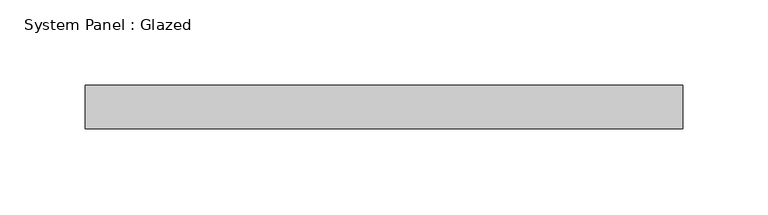
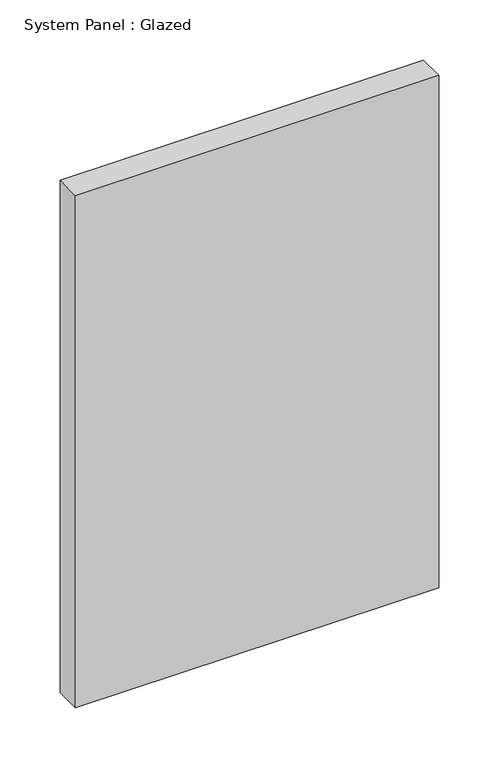
"""IFC4 building model written with IfcOpenShell, lengths in millimetres: plate geometry, System Panel : Glazed."""

from ifc_helpers import new_model, si_unit, origin, origin_with_axes, place, context, project, spatial, polyline, outline, extrude, source, transform, mapped, element, save


def system_panel_glazed_0d343f02(model_context):
    return source(origin(), model_context, "Body", "SweptSolid", [
        extrude(outline(polyline([(174.625, 19.05), (-174.625, 19.05), (-174.625, 44.45), (174.625, 44.45), (174.625, 19.05)])), origin_with_axes(), (0.0, 0.0, 1.0), 520.820328),
    ])


if __name__ == "__main__":
    model = new_model("IFC4")
    model_context = context("Model", 3, world=origin())
    ifc_project = project(units=[si_unit("LENGTHUNIT", "METRE", prefix="MILLI")], contexts=[model_context])
    site = spatial("IfcSite", under=ifc_project)
    building = spatial("IfcBuilding", under=site)
    placement = place(None, origin())
    system_panel_glazed_shape = system_panel_glazed_0d343f02(model_context)
    element("IfcPlate", 1, ObjectType="System Panel : Glazed", at=placement, inside=building, context=model_context, shape_type="MappedRepresentation", body=[
        mapped(system_panel_glazed_shape, transform((0.0, 0.0, 0.0), x_axis=(1.0, 0.0, 0.0), y_axis=(0.0, 1.0, 0.0), z_axis=(0.0, 0.0, 1.0))),
    ])
    save(model, "model.ifc")

# Revit data of these elements
# Type "System Panel : Glazed"
#   Construction Type Id = "GSP4R"
#   Analytic Construction = "1/8 in Pilkington single glazing"
#   Visual Light Transmittance = 0.9
#   Solar Heat Gain Coefficient = 0.86
#   Heat Transfer Coefficient (U) = 1.18115 BTU/(h·ft²·°F)
#   Define Thermal Properties by = 1
# Element 1 (IfcPlate, "System Panel : Glazed")
#   Materials on its faces: "Glass"
# Materials
#   "Glass": class "Glass", colour RGB 0 128 192, transparency 0.75, Description = "Soda Lime Glass", Cost = 0
